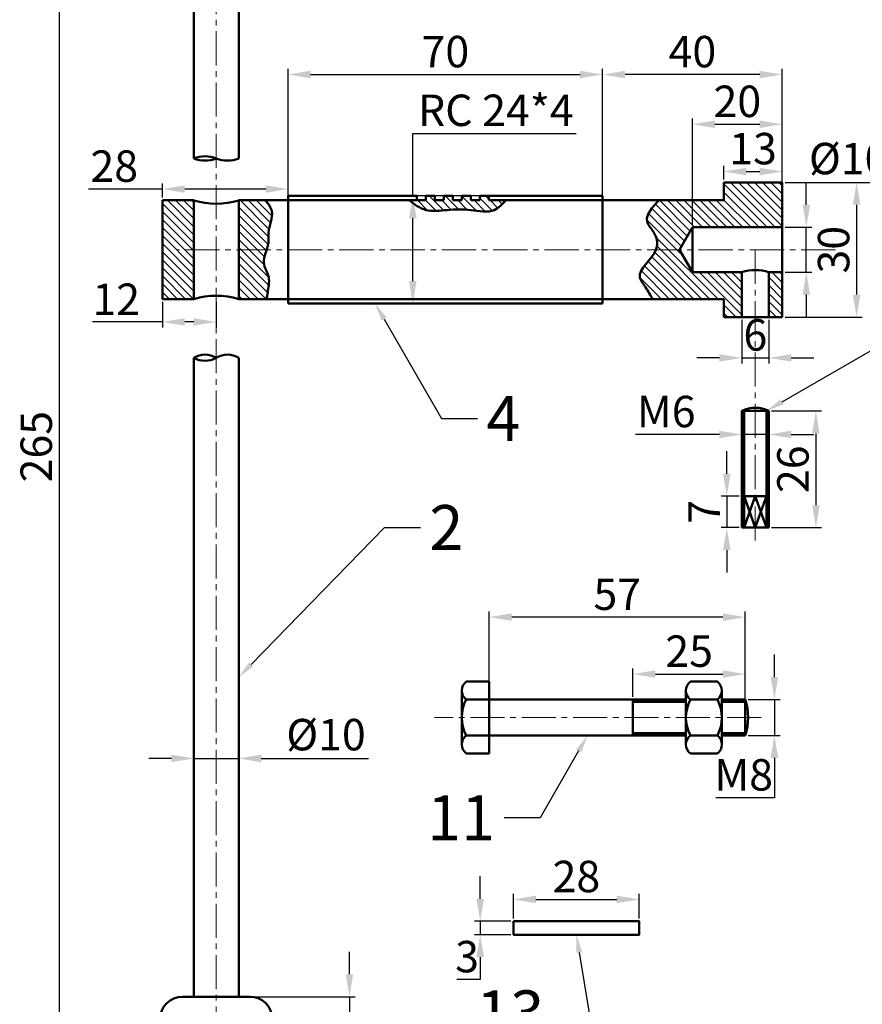
# Model space of a CAD drawing. Units: millimetres. Extents: x 434 to 1535, y -197 to 318.
# Tile 5 of 9: x 732 to 920, y -24 to 195. Entities that reach past the tile are written whole.
import ezdxf
from ezdxf import colors
from ezdxf.entities.mleader import LeaderData, LeaderLine
from ezdxf.math import Vec2, Vec3

# ---------------------------------------------------------------- set-up
doc = ezdxf.new("R2010")
doc.units = ezdxf.units.MM
doc.header["$LTSCALE"] = 0.4
doc.linetypes.add('CENTER2', pattern=[28.575, 19.05, -3.175, 3.175, -3.175])
for name, color, linetype, lineweight in [('M-CNTR', 1, 'CENTER2', 18), ('M-DIMS', 2, 'Continuous', 25), ('M-HATC', 8, 'Continuous', 18), ('M-OUTL', 7, 'Continuous', 50), ('M-TEXT', 3, 'Continuous', 25)]:
    doc.layers.add(name, color=color, linetype=linetype, lineweight=lineweight)
doc.styles.get("Standard").update_dxf_attribs({"font": 'arial.ttf'})
doc.dimstyles.new('ISO-25', dxfattribs={"dimtxt": 7, "dimasz": 5, "dimexe": 1.25, "dimexo": 0.625, "dimtad": 1, "dimtoh": 1, "dimdec": 0, "dimtxsty": 'Standard', "dimcen": 2.5, "dimadec": 0, "dimazin": 0, "dimtfac": 1, "dimtdec": 0, "dimtmove": 0, "dimatfit": 3, "dimfxl": 1, "dimarcsym": 0})
pattern_1 = [(135, (-18.9852, -70.3126), (-0.8980256, -0.8980256), [])]

# ---------------------------------------------------------------- blocks, each defined once
blk = doc.blocks.new('*U44')
at = {"layer": 'M-CNTR', "color": 0, "transparency": 16777216}
blk.add_line((62.18, 0), (-84.48, 0), dxfattribs=at)
blk = doc.blocks.new('*U45')
at = {"layer": 'M-CNTR', "color": 0, "transparency": 16777216}
blk.add_line((0, 35.41), (0, -30.04), dxfattribs=at)
blk = doc.blocks.new('*U48')
at = {"layer": 'M-CNTR', "color": 0, "transparency": 16777216}
blk.add_line((0, 223.89), (0, -74.65), dxfattribs=at)
blk = doc.blocks.new('*D53')
at = {"layer": 'Defpoints', "color": 0, "ltscale": 0.4, "transparency": 16777216}
for p in [(770.74, 232.87), (740.77, -32.13), (770.74, -32.13)]:
    blk.add_point(p, dxfattribs=at)
at = {"layer": 'M-DIMS', "color": 0, "lineweight": -2, "ltscale": 0.4, "transparency": 16777216}
for p, q in [((770.11, 232.87), (739.52, 232.87)), ((740.77, 227.87), (740.77, -27.13)), ((770.11, -32.13), (739.52, -32.13))]:
    blk.add_line(p, q, dxfattribs=at)
at = {"layer": 'M-DIMS', "color": 0, "ltscale": 0.4, "transparency": 16777216}
for points in [[(739.94, 227.87), (741.61, 227.87), (740.77, 232.87)], [(739.94, -27.13), (741.61, -27.13), (740.77, -32.13)]]:
    blk.add_solid(points, dxfattribs=at)
at = {"layer": 'M-DIMS', "color": 0, "ltscale": 0.4, "transparency": 16777216, "insert": (736.57, 100.37), "char_height": 7, "attachment_point": 5, "rotation": 90}
blk.add_mtext('265', dxfattribs=at)
blk = doc.blocks.new('*D55')
at = {"layer": 'Defpoints', "color": 0, "ltscale": 0.4, "transparency": 16777216}
for p in [(791.74, 157.73), (763.74, 155.22), (791.74, 155.22)]:
    blk.add_point(p, dxfattribs=at)
at = {"layer": 'M-DIMS', "color": 0, "lineweight": -2, "ltscale": 0.4, "transparency": 16777216}
for p, q in [((763.74, 155.84), (763.74, 158.98)), ((791.74, 155.84), (791.74, 158.98)), ((763.74, 157.73), (747.33, 157.73)), ((786.74, 157.73), (768.74, 157.73))]:
    blk.add_line(p, q, dxfattribs=at)
at = {"layer": 'M-DIMS', "color": 0, "ltscale": 0.4, "transparency": 16777216}
for points in [[(768.74, 158.57), (768.74, 156.9), (763.74, 157.73)], [(786.74, 158.57), (786.74, 156.9), (791.74, 157.73)]]:
    blk.add_solid(points, dxfattribs=at)
at = {"layer": 'M-DIMS', "color": 0, "ltscale": 0.4, "transparency": 16777216, "insert": (753.03, 161.93), "char_height": 7, "attachment_point": 5}
blk.add_mtext('28', dxfattribs=at)
blk = doc.blocks.new('*D56')
at = {"layer": 'Defpoints', "color": 0, "ltscale": 0.4, "transparency": 16777216}
for p in [(763.74, 133.22), (775.74, 133.22), (775.74, 128.14)]:
    blk.add_point(p, dxfattribs=at)
at = {"layer": 'M-DIMS', "color": 0, "lineweight": -2, "ltscale": 0.4, "transparency": 16777216}
for p, q in [((763.74, 132.59), (763.74, 126.89)), ((775.74, 132.59), (775.74, 126.89)), ((763.74, 128.14), (748.19, 128.14)), ((770.74, 128.14), (768.74, 128.14))]:
    blk.add_line(p, q, dxfattribs=at)
at = {"layer": 'M-DIMS', "color": 0, "ltscale": 0.4, "transparency": 16777216}
for points in [[(768.74, 128.97), (768.74, 127.31), (763.74, 128.14)], [(770.74, 128.97), (770.74, 127.31), (775.74, 128.14)]]:
    blk.add_solid(points, dxfattribs=at)
at = {"layer": 'M-DIMS', "color": 0, "ltscale": 0.4, "transparency": 16777216, "insert": (753.47, 132.28), "char_height": 7, "attachment_point": 5}
blk.add_mtext('12', dxfattribs=at)
blk = doc.blocks.new('*D57')
at = {"layer": 'Defpoints', "color": 0, "ltscale": 0.4, "transparency": 16777216}
for p in [(861.74, 183.23), (791.74, 155.22), (861.74, 155.22)]:
    blk.add_point(p, dxfattribs=at)
at = {"layer": 'M-DIMS', "color": 0, "lineweight": -2, "ltscale": 0.4, "transparency": 16777216}
for p, q in [((791.74, 155.84), (791.74, 184.48)), ((861.74, 155.84), (861.74, 184.48)), ((796.74, 183.23), (856.74, 183.23))]:
    blk.add_line(p, q, dxfattribs=at)
at = {"layer": 'M-DIMS', "color": 0, "ltscale": 0.4, "transparency": 16777216}
for points in [[(796.74, 184.06), (796.74, 182.4), (791.74, 183.23)], [(856.74, 184.06), (856.74, 182.4), (861.74, 183.23)]]:
    blk.add_solid(points, dxfattribs=at)
at = {"layer": 'M-DIMS', "color": 0, "ltscale": 0.4, "transparency": 16777216, "insert": (826.74, 187.43), "char_height": 7, "attachment_point": 5}
blk.add_mtext('70', dxfattribs=at)
blk = doc.blocks.new('*D58')
at = {"layer": 'Defpoints', "color": 0, "ltscale": 0.4, "transparency": 16777216}
for p in [(861.74, 183.23), (861.74, 163.37), (901.74, 159.22)]:
    blk.add_point(p, dxfattribs=at)
at = {"layer": 'M-DIMS', "color": 0, "lineweight": -2, "ltscale": 0.4, "transparency": 16777216}
for p, q in [((861.74, 163.99), (861.74, 184.48)), ((901.74, 159.84), (901.74, 184.48)), ((896.74, 183.23), (866.74, 183.23))]:
    blk.add_line(p, q, dxfattribs=at)
at = {"layer": 'M-DIMS', "color": 0, "ltscale": 0.4, "transparency": 16777216}
for points in [[(866.74, 184.06), (866.74, 182.4), (861.74, 183.23)], [(896.74, 184.06), (896.74, 182.4), (901.74, 183.23)]]:
    blk.add_solid(points, dxfattribs=at)
at = {"layer": 'M-DIMS', "color": 0, "ltscale": 0.4, "transparency": 16777216, "insert": (881.74, 187.43), "char_height": 7, "attachment_point": 5}
blk.add_mtext('40', dxfattribs=at)
blk = doc.blocks.new('*D59')
at = {"layer": 'Defpoints', "color": 0, "ltscale": 0.4, "transparency": 16777216}
for p in [(901.74, 172.16), (881.74, 149.22), (901.74, 149.22)]:
    blk.add_point(p, dxfattribs=at)
at = {"layer": 'M-DIMS', "color": 0, "lineweight": -2, "ltscale": 0.4, "transparency": 16777216}
for p, q in [((881.74, 149.84), (881.74, 173.41)), ((901.74, 149.84), (901.74, 173.41)), ((886.74, 172.16), (896.74, 172.16))]:
    blk.add_line(p, q, dxfattribs=at)
at = {"layer": 'M-DIMS', "color": 0, "ltscale": 0.4, "transparency": 16777216}
for points in [[(886.74, 172.99), (886.74, 171.33), (881.74, 172.16)], [(896.74, 172.99), (896.74, 171.33), (901.74, 172.16)]]:
    blk.add_solid(points, dxfattribs=at)
at = {"layer": 'M-DIMS', "color": 0, "ltscale": 0.4, "transparency": 16777216, "insert": (891.74, 176.36), "char_height": 7, "attachment_point": 5}
blk.add_mtext('20', dxfattribs=at)
blk = doc.blocks.new('*D60')
at = {"layer": 'Defpoints', "color": 0, "ltscale": 0.4, "transparency": 16777216}
for p in [(901.74, 161.63), (888.74, 159.22), (901.74, 159.22)]:
    blk.add_point(p, dxfattribs=at)
at = {"layer": 'M-DIMS', "color": 0, "lineweight": -2, "ltscale": 0.4, "transparency": 16777216}
for p, q in [((888.74, 159.84), (888.74, 162.88)), ((901.74, 159.84), (901.74, 162.88)), ((893.74, 161.63), (896.74, 161.63))]:
    blk.add_line(p, q, dxfattribs=at)
at = {"layer": 'M-DIMS', "color": 0, "ltscale": 0.4, "transparency": 16777216}
for points in [[(893.74, 162.46), (893.74, 160.79), (888.74, 161.63)], [(896.74, 162.46), (896.74, 160.79), (901.74, 161.63)]]:
    blk.add_solid(points, dxfattribs=at)
at = {"layer": 'M-DIMS', "color": 0, "ltscale": 0.4, "transparency": 16777216, "insert": (895.24, 165.83), "char_height": 7, "attachment_point": 5}
blk.add_mtext('13', dxfattribs=at)
blk = doc.blocks.new('*D61')
at = {"layer": 'Defpoints', "color": 0, "ltscale": 0.4, "transparency": 16777216}
for p in [(901.74, 149.22), (901.74, 139.22), (907.09, 139.22)]:
    blk.add_point(p, dxfattribs=at)
at = {"layer": 'M-DIMS', "color": 0, "lineweight": -2, "ltscale": 0.4, "transparency": 16777216}
for p, q in [((907.09, 154.22), (907.09, 159.22)), ((907.09, 159.22), (925.34, 159.22)), ((902.36, 149.22), (908.34, 149.22)), ((907.09, 139.22), (907.09, 149.22)), ((902.36, 139.22), (908.34, 139.22)), ((907.09, 134.22), (907.09, 129.22))]:
    blk.add_line(p, q, dxfattribs=at)
at = {"layer": 'M-DIMS', "color": 0, "ltscale": 0.4, "transparency": 16777216}
for points in [[(906.26, 154.22), (907.93, 154.22), (907.09, 149.22)], [(906.26, 134.22), (907.93, 134.22), (907.09, 139.22)]]:
    blk.add_solid(points, dxfattribs=at)
at = {"layer": 'M-DIMS', "color": 0, "ltscale": 0.4, "transparency": 16777216, "insert": (916.53, 163.61), "char_height": 7, "attachment_point": 5}
blk.add_mtext('%%C10', dxfattribs=at)
blk = doc.blocks.new('*D62')
at = {"layer": 'Defpoints', "color": 0, "ltscale": 0.4, "transparency": 16777216}
for p in [(901.74, 159.22), (901.74, 129.22), (918.29, 129.22)]:
    blk.add_point(p, dxfattribs=at)
at = {"layer": 'M-DIMS', "color": 0, "lineweight": -2, "ltscale": 0.4, "transparency": 16777216}
for p, q in [((902.36, 159.22), (919.54, 159.22)), ((918.29, 154.22), (918.29, 134.22)), ((902.36, 129.22), (919.54, 129.22))]:
    blk.add_line(p, q, dxfattribs=at)
at = {"layer": 'M-DIMS', "color": 0, "ltscale": 0.4, "transparency": 16777216}
for points in [[(917.45, 154.22), (919.12, 154.22), (918.29, 159.22)], [(917.45, 134.22), (919.12, 134.22), (918.29, 129.22)]]:
    blk.add_solid(points, dxfattribs=at)
at = {"layer": 'M-DIMS', "color": 0, "ltscale": 0.4, "transparency": 16777216, "insert": (914.08, 144.22), "char_height": 7, "attachment_point": 5, "rotation": 90}
blk.add_mtext('30', dxfattribs=at)
blk = doc.blocks.new('*D63')
at = {"layer": 'Defpoints', "color": 0, "ltscale": 0.4, "transparency": 16777216}
for p in [(892.74, 129.22), (898.74, 129.22), (898.74, 120.14)]:
    blk.add_point(p, dxfattribs=at)
at = {"layer": 'M-DIMS', "color": 0, "lineweight": -2, "ltscale": 0.4, "transparency": 16777216}
for p, q in [((892.74, 128.59), (892.74, 118.89)), ((898.74, 128.59), (898.74, 118.89)), ((887.74, 120.14), (882.74, 120.14)), ((892.74, 120.14), (898.74, 120.14)), ((903.74, 120.14), (908.74, 120.14))]:
    blk.add_line(p, q, dxfattribs=at)
at = {"layer": 'M-DIMS', "color": 0, "ltscale": 0.4, "transparency": 16777216}
for points in [[(887.74, 120.97), (887.74, 119.31), (892.74, 120.14)], [(903.74, 120.97), (903.74, 119.31), (898.74, 120.14)]]:
    blk.add_solid(points, dxfattribs=at)
at = {"layer": 'M-DIMS', "color": 0, "ltscale": 0.4, "transparency": 16777216, "insert": (895.74, 124.34), "char_height": 7, "attachment_point": 5}
blk.add_mtext('6', dxfattribs=at)
blk = doc.blocks.new('*D64')
at = {"layer": 'Defpoints', "color": 0, "ltscale": 0.4, "transparency": 16777216}
for p in [(898.74, 103.08), (892.74, 98.29), (898.74, 98.29)]:
    blk.add_point(p, dxfattribs=at)
at = {"layer": 'M-DIMS', "color": 0, "lineweight": -2, "ltscale": 0.4, "transparency": 16777216}
for p, q in [((887.74, 103.08), (869.08, 103.08)), ((892.74, 98.91), (892.74, 104.33)), ((898.74, 103.08), (892.74, 103.08)), ((898.74, 98.91), (898.74, 104.33)), ((903.74, 103.08), (908.74, 103.08))]:
    blk.add_line(p, q, dxfattribs=at)
at = {"layer": 'M-DIMS', "color": 0, "ltscale": 0.4, "transparency": 16777216}
for points in [[(887.74, 103.91), (887.74, 102.25), (892.74, 103.08)], [(903.74, 103.91), (903.74, 102.25), (898.74, 103.08)]]:
    blk.add_solid(points, dxfattribs=at)
at = {"layer": 'M-DIMS', "color": 0, "ltscale": 0.4, "transparency": 16777216, "insert": (875.91, 107.28), "char_height": 7, "attachment_point": 5}
blk.add_mtext('M6', dxfattribs=at)
blk = doc.blocks.new('*D65')
at = {"layer": 'Defpoints', "color": 0, "ltscale": 0.4, "transparency": 16777216}
for p in [(898.74, 108.33), (898.74, 82.33), (909.22, 82.33)]:
    blk.add_point(p, dxfattribs=at)
at = {"layer": 'M-DIMS', "color": 0, "lineweight": -2, "ltscale": 0.4, "transparency": 16777216}
for p, q in [((899.36, 108.33), (910.47, 108.33)), ((909.22, 103.33), (909.22, 87.33)), ((899.36, 82.33), (910.47, 82.33))]:
    blk.add_line(p, q, dxfattribs=at)
at = {"layer": 'M-DIMS', "color": 0, "ltscale": 0.4, "transparency": 16777216}
for points in [[(908.39, 103.33), (910.06, 103.33), (909.22, 108.33)], [(908.39, 87.33), (910.06, 87.33), (909.22, 82.33)]]:
    blk.add_solid(points, dxfattribs=at)
at = {"layer": 'M-DIMS', "color": 0, "ltscale": 0.4, "transparency": 16777216, "insert": (905.02, 95.33), "char_height": 7, "attachment_point": 5, "rotation": 90}
blk.add_mtext('26', dxfattribs=at)
blk = doc.blocks.new('*D66')
at = {"layer": 'Defpoints', "color": 0, "ltscale": 0.4, "transparency": 16777216}
for p in [(892.74, 89.33), (889.39, 82.33), (892.74, 82.33)]:
    blk.add_point(p, dxfattribs=at)
at = {"layer": 'M-DIMS', "color": 0, "lineweight": -2, "ltscale": 0.4, "transparency": 16777216}
for p, q in [((889.39, 94.33), (889.39, 99.33)), ((892.11, 89.33), (888.14, 89.33)), ((889.39, 89.33), (889.39, 82.33)), ((892.11, 82.33), (888.14, 82.33)), ((889.39, 77.33), (889.39, 72.33))]:
    blk.add_line(p, q, dxfattribs=at)
at = {"layer": 'M-DIMS', "color": 0, "ltscale": 0.4, "transparency": 16777216}
for points in [[(888.56, 94.33), (890.22, 94.33), (889.39, 89.33)], [(888.56, 77.33), (890.22, 77.33), (889.39, 82.33)]]:
    blk.add_solid(points, dxfattribs=at)
at = {"layer": 'M-DIMS', "color": 0, "ltscale": 0.4, "transparency": 16777216, "insert": (885.27, 85.83), "char_height": 7, "attachment_point": 5, "rotation": 90}
blk.add_mtext('7', dxfattribs=at)
blk = doc.blocks.new('*D67')
at = {"layer": 'Defpoints', "color": 0, "ltscale": 0.4, "transparency": 16777216}
for p in [(848.08, 156.22), (819.49, 132.22), (848.08, 132.22)]:
    blk.add_point(p, dxfattribs=at)
at = {"layer": 'M-DIMS', "color": 0, "lineweight": -2, "ltscale": 0.4, "transparency": 16777216}
for p, q in [((819.49, 156.22), (819.49, 170.11)), ((819.49, 170.11), (855.83, 170.11)), ((847.46, 156.22), (818.24, 156.22)), ((819.49, 137.22), (819.49, 151.22)), ((847.46, 132.22), (818.24, 132.22))]:
    blk.add_line(p, q, dxfattribs=at)
at = {"layer": 'M-DIMS', "color": 0, "ltscale": 0.4, "transparency": 16777216}
for points in [[(818.65, 151.22), (820.32, 151.22), (819.49, 156.22)], [(818.65, 137.22), (820.32, 137.22), (819.49, 132.22)]]:
    blk.add_solid(points, dxfattribs=at)
at = {"layer": 'M-DIMS', "color": 0, "ltscale": 0.4, "transparency": 16777216, "insert": (837.97, 174.36), "char_height": 7, "attachment_point": 5}
blk.add_mtext('RC 24*4', dxfattribs=at)
blk = doc.blocks.new('*D68')
at = {"layer": 'Defpoints', "color": 0, "ltscale": 0.4, "transparency": 16777216}
for p in [(775.74, -22.13), (775.74, -32.13), (805.39, -32.13)]:
    blk.add_point(p, dxfattribs=at)
at = {"layer": 'M-DIMS', "color": 0, "lineweight": -2, "ltscale": 0.4, "transparency": 16777216}
for p, q in [((805.39, -17.13), (805.39, -12.13)), ((776.36, -22.13), (806.64, -22.13)), ((805.39, -22.13), (805.39, -32.13)), ((776.36, -32.13), (806.64, -32.13)), ((805.39, -37.13), (805.39, -42.13)), ((805.39, -42.13), (795.42, -42.13))]:
    blk.add_line(p, q, dxfattribs=at)
at = {"layer": 'M-DIMS', "color": 0, "ltscale": 0.4, "transparency": 16777216}
for points in [[(804.55, -17.13), (806.22, -17.13), (805.39, -22.13)], [(804.55, -37.13), (806.22, -37.13), (805.39, -32.13)]]:
    blk.add_solid(points, dxfattribs=at)
at = {"layer": 'M-DIMS', "color": 0, "ltscale": 0.4, "transparency": 16777216, "insert": (800.09, -37.93), "char_height": 7, "attachment_point": 5}
blk.add_mtext('10', dxfattribs=at)
blk = doc.blocks.new('*D69')
at = {"layer": 'Defpoints', "color": 0, "ltscale": 0.4, "transparency": 16777216}
for p in [(770.74, 30.94), (780.74, 30.94), (780.74, 30.94)]:
    blk.add_point(p, dxfattribs=at)
at = {"layer": 'M-DIMS', "color": 0, "lineweight": -2, "ltscale": 0.4, "transparency": 16777216}
for p, q in [((765.74, 30.94), (760.74, 30.94)), ((770.74, 31.56), (770.74, 32.19)), ((770.74, 30.94), (780.74, 30.94)), ((780.74, 31.56), (780.74, 32.19)), ((785.74, 30.94), (809.61, 30.94))]:
    blk.add_line(p, q, dxfattribs=at)
at = {"layer": 'M-DIMS', "color": 0, "ltscale": 0.4, "transparency": 16777216}
for points in [[(765.74, 31.77), (765.74, 30.1), (770.74, 30.94)], [(785.74, 31.77), (785.74, 30.1), (780.74, 30.94)]]:
    blk.add_solid(points, dxfattribs=at)
at = {"layer": 'M-DIMS', "color": 0, "ltscale": 0.4, "transparency": 16777216, "insert": (800.17, 35.33), "char_height": 7, "attachment_point": 5}
blk.add_mtext('%%C10', dxfattribs=at)
blk = doc.blocks.new('*U70')
at = {"layer": 'M-CNTR', "color": 0, "transparency": 16777216}
blk.add_line((22.42, 0), (-50.3, 0), dxfattribs=at)
blk = doc.blocks.new('*D71')
at = {"layer": 'Defpoints', "color": 0, "ltscale": 0.4, "transparency": 16777216}
for p in [(836.51, 62.4), (893.51, 41.74), (836.51, 40.06)]:
    blk.add_point(p, dxfattribs=at)
at = {"layer": 'M-DIMS', "color": 0, "lineweight": -2, "ltscale": 0.4, "transparency": 16777216}
for p, q in [((836.51, 40.68), (836.51, 63.65)), ((893.51, 42.36), (893.51, 63.65)), ((888.51, 62.4), (841.51, 62.4))]:
    blk.add_line(p, q, dxfattribs=at)
at = {"layer": 'M-DIMS', "color": 0, "ltscale": 0.4, "transparency": 16777216}
for points in [[(841.51, 63.24), (841.51, 61.57), (836.51, 62.4)], [(888.51, 63.24), (888.51, 61.57), (893.51, 62.4)]]:
    blk.add_solid(points, dxfattribs=at)
at = {"layer": 'M-DIMS', "color": 0, "ltscale": 0.4, "transparency": 16777216, "insert": (865.01, 66.59), "char_height": 7, "attachment_point": 5}
blk.add_mtext('57', dxfattribs=at)
blk = doc.blocks.new('*D72')
at = {"layer": 'Defpoints', "color": 0, "ltscale": 0.4, "transparency": 16777216}
for p in [(893.51, 49.73), (868.51, 44.06), (893.51, 40.06)]:
    blk.add_point(p, dxfattribs=at)
at = {"layer": 'M-DIMS', "color": 0, "lineweight": -2, "ltscale": 0.4, "transparency": 16777216}
for p, q in [((868.51, 44.68), (868.51, 50.98)), ((893.51, 40.68), (893.51, 50.98)), ((873.51, 49.73), (888.51, 49.73))]:
    blk.add_line(p, q, dxfattribs=at)
at = {"layer": 'M-DIMS', "color": 0, "ltscale": 0.4, "transparency": 16777216}
for points in [[(873.51, 50.56), (873.51, 48.89), (868.51, 49.73)], [(888.51, 50.56), (888.51, 48.89), (893.51, 49.73)]]:
    blk.add_solid(points, dxfattribs=at)
at = {"layer": 'M-DIMS', "color": 0, "ltscale": 0.4, "transparency": 16777216, "insert": (881.01, 53.92), "char_height": 7, "attachment_point": 5}
blk.add_mtext('25', dxfattribs=at)
blk = doc.blocks.new('*D73')
at = {"layer": 'Defpoints', "color": 0, "ltscale": 0.4, "transparency": 16777216}
for p in [(893.51, 44.06), (893.51, 36.06), (899.99, 36.06)]:
    blk.add_point(p, dxfattribs=at)
at = {"layer": 'M-DIMS', "color": 0, "lineweight": -2, "ltscale": 0.4, "transparency": 16777216}
for p, q in [((899.99, 49.06), (899.99, 54.06)), ((894.13, 44.06), (901.24, 44.06)), ((899.99, 44.06), (899.99, 36.06)), ((894.13, 36.06), (901.24, 36.06)), ((899.99, 31.06), (899.99, 22.18)), ((899.99, 22.18), (886.94, 22.18))]:
    blk.add_line(p, q, dxfattribs=at)
at = {"layer": 'M-DIMS', "color": 0, "ltscale": 0.4, "transparency": 16777216}
for points in [[(899.16, 49.06), (900.83, 49.06), (899.99, 44.06)], [(899.16, 31.06), (900.83, 31.06), (899.99, 36.06)]]:
    blk.add_solid(points, dxfattribs=at)
at = {"layer": 'M-DIMS', "color": 0, "ltscale": 0.4, "transparency": 16777216, "insert": (893.15, 26.38), "char_height": 7, "attachment_point": 5}
blk.add_mtext('M8', dxfattribs=at)
blk = doc.blocks.new('*D74')
at = {"layer": 'Defpoints', "color": 0, "ltscale": 0.4, "transparency": 16777216}
for p in [(841.91, -5.31), (834.5, -8.31), (841.91, -8.31)]:
    blk.add_point(p, dxfattribs=at)
at = {"layer": 'M-DIMS', "color": 0, "lineweight": -2, "ltscale": 0.4, "transparency": 16777216}
for p, q in [((834.5, -0.31), (834.5, 4.69)), ((841.29, -5.31), (833.25, -5.31)), ((834.5, -5.31), (834.5, -8.31)), ((841.29, -8.31), (833.25, -8.31)), ((834.5, -13.31), (834.5, -18.31)), ((834.5, -18.31), (829.29, -18.31))]:
    blk.add_line(p, q, dxfattribs=at)
at = {"layer": 'M-DIMS', "color": 0, "ltscale": 0.4, "transparency": 16777216}
for points in [[(833.67, -0.31), (835.33, -0.31), (834.5, -5.31)], [(833.67, -13.31), (835.33, -13.31), (834.5, -8.31)]]:
    blk.add_solid(points, dxfattribs=at)
at = {"layer": 'M-DIMS', "color": 0, "ltscale": 0.4, "transparency": 16777216, "insert": (831.58, -14.11), "char_height": 7, "attachment_point": 5}
blk.add_mtext('3', dxfattribs=at)
blk = doc.blocks.new('*D75')
at = {"layer": 'Defpoints', "color": 0, "ltscale": 0.4, "transparency": 16777216}
for p in [(869.91, -0.46), (841.91, -5.31), (869.91, -5.31)]:
    blk.add_point(p, dxfattribs=at)
at = {"layer": 'M-DIMS', "color": 0, "lineweight": -2, "ltscale": 0.4, "transparency": 16777216}
for p, q in [((841.91, -4.68), (841.91, 0.79)), ((869.91, -4.68), (869.91, 0.79)), ((846.91, -0.46), (864.91, -0.46))]:
    blk.add_line(p, q, dxfattribs=at)
at = {"layer": 'M-DIMS', "color": 0, "ltscale": 0.4, "transparency": 16777216}
for points in [[(846.91, 0.37), (846.91, -1.29), (841.91, -0.46)], [(864.91, 0.37), (864.91, -1.29), (869.91, -0.46)]]:
    blk.add_solid(points, dxfattribs=at)
at = {"layer": 'M-DIMS', "color": 0, "ltscale": 0.4, "transparency": 16777216, "insert": (855.91, 3.74), "char_height": 7, "attachment_point": 5}
blk.add_mtext('28', dxfattribs=at)

msp = doc.modelspace()

# ---------------------------------------------------------------- hatches: boundary and pattern name
at = {"layer": 'M-HATC', "ltscale": 0.4}
h = msp.add_hatch(dxfattribs=at)
h.set_pattern_fill('ANSI31', color=256, scale=0.4, angle=90)
h.set_pattern_definition(pattern_1)
edge = h.paths.add_edge_path()
edge.add_line((888.74, 155.22), (874.31, 155.22))
edge.add_spline(control_points=[(874.31, 155.22), (872.82, 153.65), (870.22, 150.92), (874.02, 147.63), (874.01, 145.17), (873.63, 144.22)], knot_values=[0, 0, 0, 0, 5.334799, 9.307994, 12.247035, 12.247035, 12.247035, 12.247035], degree=3, periodic=0)
edge.add_line((873.63, 144.22), (878.85, 144.22))
edge.add_line((878.85, 144.22), (881.74, 149.22))
edge.add_line((881.74, 149.22), (901.74, 149.22))
edge.add_line((901.74, 149.22), (901.74, 159.22))
edge.add_line((901.74, 159.22), (888.74, 159.22))
edge.add_line((888.74, 159.22), (888.74, 155.22))
edge = h.paths.add_edge_path()
edge.add_line((888.74, 133.22), (888.74, 129.22))
edge.add_line((888.74, 129.22), (892.74, 129.22))
edge.add_line((892.74, 129.22), (892.74, 139.22))
edge.add_line((892.74, 139.22), (881.74, 139.22))
edge.add_line((881.74, 139.22), (878.85, 144.22))
edge.add_line((878.85, 144.22), (873.63, 144.22))
edge.add_spline(control_points=[(873.63, 144.22), (872.72, 141.89), (868.52, 139.41), (871.55, 135.69), (872.39, 134.09), (872.85, 133.22)], knot_values=[12.247035, 12.247035, 12.247035, 12.247035, 19.381632, 21.904984, 24.948741, 24.948741, 24.948741, 24.948741], degree=3, periodic=0)
edge.add_line((872.85, 133.22), (888.74, 133.22))
h.paths.add_polyline_path([(901.74, 139.22), (898.74, 139.22), (898.74, 129.22), (901.74, 129.22)])
h = msp.add_hatch(dxfattribs=at)
h.set_pattern_fill('ANSI31', color=256, scale=0.4, angle=90)
h.set_pattern_definition(pattern_1)
h.paths.add_polyline_path([(770.74, 155.22), (763.74, 155.22), (763.74, 133.22), (770.74, 133.22)])
edge = h.paths.add_edge_path()
edge.add_line((780.74, 144.22), (786.97, 144.22))
edge.add_spline(control_points=[(786.97, 144.22), (787.14, 144.72), (787.52, 145.97), (787, 148.85), (788.99, 152.29), (787.33, 154.43), (786.73, 155.22)], knot_values=[0, 0, 0, 0, 1.52572, 3.813757, 8.665239, 11.451838, 11.451838, 11.451838, 11.451838], degree=3, periodic=0)
edge.add_line((786.73, 155.22), (780.74, 155.22))
edge.add_line((780.74, 155.22), (780.74, 144.22))
edge = h.paths.add_edge_path()
edge.add_line((780.74, 144.22), (780.74, 133.22))
edge.add_line((780.74, 133.22), (786.9, 133.22))
edge.add_spline(control_points=[(786.9, 133.22), (787.1, 134.24), (787.41, 135.84), (787.61, 138.65), (785.73, 141.14), (786.63, 143.22), (786.97, 144.22)], knot_values=[11.451838, 11.451838, 11.451838, 11.451838, 14.589724, 16.361749, 19.755155, 22.78424, 22.78424, 22.78424, 22.78424], degree=3, periodic=0)
edge.add_line((786.97, 144.22), (780.74, 144.22))
edge = h.paths.add_edge_path()
edge.add_line((834.42, 155.22), (832.42, 155.22))
edge.add_line((832.42, 155.22), (832.42, 156.22))
edge.add_line((832.42, 156.22), (830.42, 156.22))
edge.add_line((830.42, 156.22), (830.42, 155.22))
edge.add_line((830.42, 155.22), (828.42, 155.22))
edge.add_line((828.42, 155.22), (828.42, 156.22))
edge.add_line((828.42, 156.22), (826.42, 156.22))
edge.add_line((826.42, 156.22), (826.42, 155.22))
edge.add_line((826.42, 155.22), (824.42, 155.22))
edge.add_line((824.42, 155.22), (824.42, 156.22))
edge.add_line((824.42, 156.22), (822.42, 156.22))
edge.add_line((822.42, 156.22), (822.42, 155.22))
edge.add_line((822.42, 155.22), (820.42, 155.22))
edge.add_line((820.42, 155.22), (818.68, 155.22))
edge.add_spline(control_points=[(818.68, 155.22), (819.88, 154.32), (822.38, 152.44), (827.41, 153.19), (832.28, 153.3), (837.36, 152.13), (839.43, 154.34), (840.24, 155.22)], knot_values=[0, 0, 0, 0, 4.313954, 9.046043, 14.31639, 19.527519, 22.91005, 22.91005, 22.91005, 22.91005], degree=3, periodic=0)
edge.add_line((840.24, 155.22), (836.42, 155.22))
edge.add_line((836.42, 155.22), (836.42, 156.22))
edge.add_line((836.42, 156.22), (834.42, 156.22))
edge.add_line((834.42, 156.22), (834.42, 155.22))

# ---------------------------------------------------------------- linework, layer by layer
at = {"layer": 'M-OUTL', "ltscale": 0.4}
for p, q in [((770.74, 232.87), (770.74, 164.55)), ((780.74, 232.87), (780.74, 164.55)), ((901.74, 159.22), (888.74, 159.22)), ((888.74, 159.22), (888.74, 155.22)), ((901.74, 144.22), (901.74, 159.22)), ((791.74, 156.22), (791.74, 132.22)), ((820.42, 156.22), (791.74, 156.22)), ((820.42, 156.22), (820.42, 155.22)), ((822.42, 155.22), (822.42, 156.22)), ((824.42, 156.22), (822.42, 156.22)), ((824.42, 156.22), (824.42, 155.22)), ((826.42, 155.22), (826.42, 156.22)), ((826.42, 156.22), (828.42, 156.22)), ((828.42, 156.22), (826.42, 156.22)), ((828.42, 156.22), (828.42, 155.22)), ((830.42, 155.22), (830.42, 156.22)), ((830.42, 156.22), (832.42, 156.22)), ((832.42, 156.22), (830.42, 156.22)), ((832.42, 156.22), (832.42, 155.22)), ((861.74, 156.22), (834.42, 156.22)), ((834.42, 155.22), (834.42, 156.22)), ((834.42, 156.22), (836.42, 156.22)), ((836.42, 156.22), (836.42, 155.22)), ((861.74, 132.22), (861.74, 156.22)), ((763.74, 155.22), (763.74, 133.22)), ((770.74, 155.22), (763.74, 155.22)), ((770.74, 155.22), (770.74, 133.22)), ((791.74, 155.22), (780.74, 155.22)), ((780.74, 155.22), (780.74, 133.22)), ((822.42, 155.22), (791.74, 155.22)), ((820.42, 155.22), (822.42, 155.22)), ((824.42, 155.22), (826.42, 155.22)), ((826.42, 155.22), (824.42, 155.22)), ((828.42, 155.22), (830.42, 155.22)), ((830.42, 155.22), (828.42, 155.22)), ((832.42, 155.22), (834.42, 155.22)), ((834.42, 155.22), (832.42, 155.22)), ((888.74, 155.22), (836.42, 155.22)), ((881.74, 149.22), (878.85, 144.22)), ((901.74, 149.22), (881.74, 149.22)), ((881.74, 149.22), (881.74, 139.22)), ((881.74, 139.22), (878.85, 144.22)), ((901.74, 129.22), (901.74, 144.22)), ((881.74, 139.22), (892.74, 139.22)), ((892.74, 129.22), (892.74, 139.22)), ((898.74, 129.22), (898.74, 139.22)), ((898.74, 139.22), (901.74, 139.22)), ((763.74, 133.22), (770.74, 133.22)), ((780.74, 133.22), (791.74, 133.22)), ((791.74, 133.22), (888.74, 133.22)), ((791.74, 132.22), (861.74, 132.22)), ((888.74, 133.22), (888.74, 129.22)), ((888.74, 129.22), (901.74, 129.22)), ((901.74, 129.22), (895.74, 129.22)), ((770.74, 120.17), (770.74, -22.13)), ((780.74, 120.17), (780.74, -22.13)), ((898.74, 108.33), (892.74, 108.33)), ((892.74, 108.33), (892.74, 82.33)), ((893.24, 108.33), (893.24, 82.33)), ((898.24, 82.33), (898.24, 108.33)), ((898.74, 82.33), (898.74, 108.33)), ((892.74, 89.33), (898.74, 89.33)), ((893.24, 82.33), (895.74, 89.33)), ((895.74, 82.33), (893.24, 89.33)), ((895.74, 89.33), (898.24, 82.33)), ((895.74, 82.33), (898.24, 89.33)), ((892.74, 82.33), (898.74, 82.33)), ((830.4, 33.95), (830.4, 46.21)), ((831.4, 48.06), (836.51, 48.06)), ((836.51, 48.06), (836.51, 32.06)), ((880.29, 33.93), (880.29, 46.19)), ((881.29, 48.04), (887.29, 48.04)), ((888.29, 46.19), (888.29, 33.93)), ((836.51, 44.06), (831.4, 44.06)), ((836.51, 36.06), (836.51, 44.06)), ((836.51, 44.06), (880.29, 44.06)), ((868.51, 44.06), (868.51, 36.06)), ((881.27, 44.06), (887.32, 44.06)), ((888.29, 44.06), (893.51, 44.06)), ((893.51, 44.06), (893.51, 36.06)), ((868.51, 43.56), (880.29, 43.56)), ((888.29, 43.56), (893.51, 43.56)), ((836.51, 36.06), (831.4, 36.06)), ((880.29, 36.06), (836.51, 36.06)), ((880.29, 36.56), (868.51, 36.56)), ((887.3, 36.06), (881.28, 36.06)), ((893.51, 36.56), (888.29, 36.56)), ((893.51, 36.06), (888.29, 36.06)), ((836.51, 32.06), (831.4, 32.06)), ((887.29, 32.04), (881.29, 32.04))]:
    msp.add_line(p, q, dxfattribs=at)
msp.add_lwpolyline([(841.91, -5.31), (869.91, -5.31), (869.91, -8.31), (841.91, -8.31)], close=True, dxfattribs=at)
msp.add_lwpolyline([(768.24, -22.13, 1), (768.24, -32.13), (783.24, -32.13, 1), (783.24, -22.13)], format="xyb", close=True, dxfattribs=at)
for centre, radius, start, end in [((773.24, 158.43), 6.61, 67.7782, 112.2218), ((773.24, 170.67), 6.61, 247.7782, 292.2218), ((778.24, 170.67), 6.61, 247.7782, 292.2218), ((775.74, 171.46), 17, 252.8954, 287.1046), ((895.74, 130.1), 9.6, 71.7903, 108.2097), ((775.74, 116.97), 17, 72.8954, 107.1046), ((773.24, 115.99), 4.86, 59.0646, 120.9354), ((778.24, 115.99), 4.86, 59.0646, 120.9354), ((773.24, 124.34), 4.86, 239.0646, 300.9354), ((895.74, 102.38), 6.66, 63.2296, 116.7704), ((832.89, 46.06), 2.49, 126.6565, 233.3435), ((882.78, 46.04), 2.49, 126.6565, 233.3435), ((885.8, 46.04), 2.49, 306.6565, 53.3435), ((838.9, 40.06), 8.5, 151.9275, 208.0725), ((888.79, 40.04), 8.5, 151.9275, 208.0725), ((879.79, 40.04), 8.5, 331.9275, 28.0725), ((880.66, 40.06), 13.46, 342.7054, 17.2946), ((832.89, 34.06), 2.5, 126.7544, 233.2456), ((882.79, 34.04), 2.5, 126.7544, 233.2456), ((885.8, 34.04), 2.5, 306.7544, 53.2456)]:
    msp.add_arc(centre, radius, start, end, dxfattribs=at)
for points, knots in [([(786.73, 155.22), (787.33, 154.43), (788.99, 152.29), (787, 148.85), (787.7, 144.97), (785.38, 141.61), (787.61, 138.65), (787.41, 135.84), (787.1, 134.24), (786.9, 133.22)], [0, 0, 0, 0, 2.786599, 7.638081, 9.926118, 14.480923, 17.874328, 19.646354, 22.78424, 22.78424, 22.78424, 22.78424]), ([(818.68, 155.22), (819.88, 154.32), (822.38, 152.44), (827.41, 153.19), (832.28, 153.3), (837.36, 152.13), (839.43, 154.34), (840.24, 155.22)], [0, 0, 0, 0, 4.313954, 9.046043, 14.31639, 19.527519, 22.91005, 22.91005, 22.91005, 22.91005]), ([(874.31, 155.22), (872.82, 153.65), (870.22, 150.92), (874.02, 147.63), (873.99, 142.64), (868.52, 139.41), (871.55, 135.69), (872.39, 134.09), (872.85, 133.22)], [0, 0, 0, 0, 5.334799, 9.307994, 12.247035, 19.381632, 21.904984, 24.948741, 24.948741, 24.948741, 24.948741])]:
    msp.add_open_spline(points, degree=3, knots=knots, dxfattribs=at)

# ---------------------------------------------------------------- block references
at = {"layer": 'M-CNTR'}
for name, p in [('*U48', (775.74, 49.02)), ('*U44', (851.41, 144.22)), ('*U45', (895.74, 108.8)), ('*U70', (874.65, 40.06))]:
    msp.add_blockref(name, p, dxfattribs=at)

# ---------------------------------------------------------------- dimensions: what is measured, and where the dimension line sits
at = {"layer": 'M-DIMS', "ltscale": 0.4}
for base, p1, p2, picture, middle in [((740.77, -32.13), (770.74, 232.87), (770.74, -32.13), '*D53', (736.57, 100.37)), ((918.29, 129.22), (901.74, 159.22), (901.74, 129.22), '*D62', (914.08, 144.22)), ((909.22, 82.33), (898.74, 108.33), (898.74, 82.33), '*D65', (905.02, 95.33)), ((889.39, 82.33), (892.74, 89.33), (892.74, 82.33), '*D66', (885.27, 85.83)), ((834.5, -8.31), (841.91, -5.31), (841.91, -8.31), '*D74', (831.58, -14.11)), ((805.39, -32.13), (775.74, -22.13), (775.74, -32.13), '*D68', (800.09, -37.93))]:
    dim = msp.add_linear_dim(base=base, p1=p1, p2=p2, angle=90, dimstyle='ISO-25', override={"dimclrd": 0, "dimclre": 0, "dimclrt": 0}, dxfattribs=at)
    dim.commit()
    dim.dimension.update_dxf_attribs({"geometry": picture, "text_midpoint": middle})
for base, p1, p2, picture, middle in [((861.74, 183.23), (791.74, 155.22), (861.74, 155.22), '*D57', (826.74, 187.43)), ((901.74, 172.16), (881.74, 149.22), (901.74, 149.22), '*D59', (891.74, 176.36)), ((901.74, 161.63), (888.74, 159.22), (901.74, 159.22), '*D60', (895.24, 165.83)), ((898.74, 120.14), (892.74, 129.22), (898.74, 129.22), '*D63', (895.74, 124.34)), ((893.51, 49.73), (868.51, 44.06), (893.51, 40.06), '*D72', (881.01, 53.92)), ((869.91, -0.46), (841.91, -5.31), (869.91, -5.31), '*D75', (855.91, 3.74))]:
    dim = msp.add_linear_dim(base=base, p1=p1, p2=p2, dimstyle='ISO-25', override={"dimclrd": 0, "dimclre": 0, "dimclrt": 0}, dxfattribs=at)
    dim.commit()
    dim.dimension.update_dxf_attribs({"geometry": picture, "text_midpoint": middle})
for base, p1, p2, picture, middle in [((861.74, 183.23), (901.74, 159.22), (861.74, 163.37), '*D58', (881.74, 183.23)), ((791.74, 157.73), (763.74, 155.22), (791.74, 155.22), '*D55', (753.03, 157.73)), ((775.74, 128.14), (763.74, 133.22), (775.74, 133.22), '*D56', (753.47, 128.14)), ((836.51, 62.4), (893.51, 41.74), (836.51, 40.06), '*D71', (865.01, 62.4))]:
    dim = msp.add_linear_dim(base=base, p1=p1, p2=p2, dimstyle='ISO-25', override={"dimclrd": 0, "dimclre": 0, "dimclrt": 0}, dxfattribs=at)
    dim.commit()
    dim.dimension.update_dxf_attribs({"geometry": picture, "text_midpoint": middle, "dimtype": 160})
for base, p1, p2, text, picture, middle in [((819.49, 132.22), (848.08, 156.22), (848.08, 132.22), 'RC 24*4', '*D67', (837.97, 170.11)), ((907.09, 139.22), (901.74, 149.22), (901.74, 139.22), '%%C<>', '*D61', (916.53, 159.22)), ((899.99, 36.06), (893.51, 44.06), (893.51, 36.06), 'M<>', '*D73', (893.15, 22.18))]:
    dim = msp.add_linear_dim(base=base, p1=p1, p2=p2, angle=90, text=text, dimstyle='ISO-25', override={"dimclrd": 0, "dimclre": 0, "dimclrt": 0}, dxfattribs=at)
    dim.commit()
    dim.dimension.update_dxf_attribs({"geometry": picture, "text_midpoint": middle, "dimtype": 160})
dim = msp.add_linear_dim(base=(898.74, 103.08), p1=(892.74, 98.29), p2=(898.74, 98.29), text='M<>', dimstyle='ISO-25', override={"dimclrd": 0, "dimclre": 0, "dimclrt": 0}, dxfattribs=at)
dim.commit()
dim.dimension.update_dxf_attribs({"geometry": '*D64', "text_midpoint": (875.91, 103.08), "dimtype": 160})
dim = msp.add_linear_dim(base=(780.74, 30.94), p1=(770.74, 30.94), p2=(780.74, 30.94), text='%%C<>', dimstyle='ISO-25', override={"dimclrd": 0, "dimclre": 0, "dimclrt": 0}, dxfattribs=at)
dim.commit()
dim.dimension.update_dxf_attribs({"geometry": '*D69', "text_midpoint": (800.17, 35.33)})

# ---------------------------------------------------------------- leaders
at = {"layer": 'M-TEXT', "ltscale": 0.4}
ml = msp.add_multileader_mtext('Standard', dxfattribs=at)
ml.set_content('4', color=256)
ml.set_leader_properties()
ml.build(insert=Vec2(0, 0))
ctx = ml.context
ctx.base_point, ctx.char_height, ctx.plane_origin = Vec3(833.87, 106.65), 10, Vec3(811.11, 132.22)
notes = []
notes.append((ctx, [(0, (1, 1, 0), (825.87, 106.65), (1, 0), 8, [(0, [(811.11, 132.22)], 0, [])])]))
ctx.mtext.insert, ctx.mtext.flow_direction = Vec3(835.87, 111.65), 5
ml = msp.add_multileader_mtext('Standard', dxfattribs=at)
ml.set_content('5', color=256)
ml.set_leader_properties()
ml.build(insert=Vec2(0, 0))
ctx = ml.context
ctx.base_point, ctx.char_height, ctx.plane_origin = Vec3(931.47, 122.89), 10, Vec3(898.24, 108.33)
notes.append((ctx, [(0, (1, 1, 0), (923.47, 122.89), (1, 0), 8, [(0, [(898.24, 108.33)], 0, [])])]))
ctx.mtext.insert, ctx.mtext.flow_direction = Vec3(933.47, 127.98), 5
ml = msp.add_multileader_mtext('Standard', dxfattribs=at)
ml.set_content('2', color=256)
ml.set_leader_properties()
ml.build(insert=Vec2(0, 0))
ctx = ml.context
ctx.base_point, ctx.char_height, ctx.plane_origin = Vec3(821.18, 82.36), 10, Vec3(780.74, 49.02)
notes.append((ctx, [(0, (1, 1, 0), (813.18, 82.36), (1, 0), 8, [(0, [(780.74, 49.02)], 0, [])])]))
ctx.mtext.insert, ctx.mtext.flow_direction = Vec3(823.18, 87.36), 5
ml = msp.add_multileader_mtext('Standard', dxfattribs=at)
ml.set_content('11', color=256)
ml.set_leader_properties()
ml.build(insert=Vec2(0, 0))
ctx = ml.context
ctx.base_point, ctx.char_height, ctx.plane_origin = Vec3(824.37, 17.73), 10, Vec3(858.4, 36.06)
ctx.text_align_type = 2
notes.append((ctx, [(0, (1, 1, 0), (847.82, 17.73), (-1, 0), 8, [(0, [(858.4, 36.06)], 0, [])])]))
ctx.mtext.insert, ctx.mtext.alignment, ctx.mtext.flow_direction = Vec3(837.82, 22.73), 3, 5
ml = msp.add_multileader_mtext('Standard', dxfattribs=at)
ml.set_content('13', color=256)
ml.set_leader_properties()
ml.build(insert=Vec2(0, 0))
ctx = ml.context
ctx.base_point, ctx.char_height, ctx.plane_origin = Vec3(833.37, -25.8), 10, Vec3(855.91, -8.31)
ctx.text_align_type = 2
notes.append((ctx, [(0, (1, 1, 0), (858.75, -25.8), (-1, 0), 8, [(0, [(855.91, -8.31)], 0, [])])]))
ctx.mtext.insert, ctx.mtext.alignment, ctx.mtext.flow_direction = Vec3(848.75, -20.71), 3, 5
for ctx, leaders in notes:
    for number, flags, end, landing, length, lines in leaders:
        leader = LeaderData()
        leader.index, (leader.has_last_leader_line, leader.has_dogleg_vector, leader.attachment_direction) = number, flags
        leader.last_leader_point, leader.dogleg_vector, leader.dogleg_length = Vec3(end), Vec3(landing), length
        for number, points, colour, breaks in lines:
            line = LeaderLine()
            line.index, line.vertices, line.color, line.breaks = number, Vec3.list(points), colors.encode_raw_color(colour), breaks
            leader.lines.append(line)
        ctx.leaders.append(leader)

doc.saveas('drawing.dxf')
